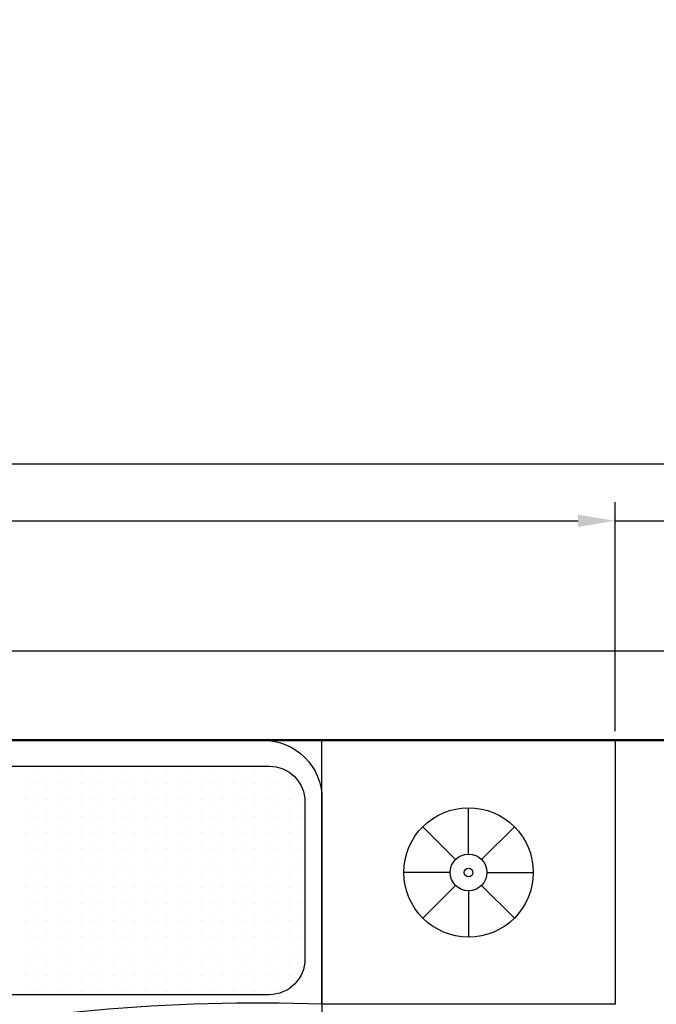
# Model space of a CAD drawing. Units: inches. Extents: x 3064 to 19385, y 846 to 15425.
# Tile 8 of 108: x 3469 to 3511, y 1373 to 1439. Entities that reach past the tile are written whole.
import ezdxf

# ---------------------------------------------------------------- set-up
doc = ezdxf.new("R2010")
doc.units = ezdxf.units.IN
for name, color, linetype, lineweight in [('A-ANNO-DIMS', 2, 'Continuous', 18), ('A-FLOR-FIXT', 9, 'Continuous', 18), ('A-WALL', 7, 'Continuous', 50), ('C-PROP', 6, 'Continuous', 25)]:
    doc.layers.add(name, color=color, linetype=linetype, lineweight=lineweight)
doc.layers.add('BLOCK', color=6, linetype='Continuous')
doc.styles.get("Standard").update_dxf_attribs({"font": 'arial.ttf'})
doc.dimstyles.new('ISO-25', dxfattribs={"dimtxt": 9, "dimasz": 2.5, "dimexe": 1.25, "dimexo": 0.625, "dimtad": 1, "dimdec": 1, "dimlunit": 3, "dimtxsty": 'Standard', "dimcen": 2.5, "dimadec": 0, "dimazin": 0, "dimtfac": 1, "dimtdec": 1, "dimtmove": 0, "dimatfit": 3, "dimfxl": 1, "dimarcsym": 0})

# ---------------------------------------------------------------- blocks, each defined once
blk = doc.blocks.new('*X7')
at = {"color": 0}
for p, q in [((275.4375, 457.03125), (275.4375, 457.03125)), ((275.625, 456.9375), (275.625, 456.9375)), ((275.8125, 457.03125), (275.8125, 457.03125)), ((276, 456.9375), (276, 456.9375)), ((276.1875, 457.03125), (276.1875, 457.03125)), ((276.375, 456.9375), (276.375, 456.9375)), ((276.5625, 457.03125), (276.5625, 457.03125)), ((276.75, 456.9375), (276.75, 456.9375)), ((276.9375, 457.03125), (276.9375, 457.03125)), ((277.125, 456.9375), (277.125, 456.9375)), ((277.3125, 457.03125), (277.3125, 457.03125)), ((277.5, 456.9375), (277.5, 456.9375)), ((277.6875, 457.03125), (277.6875, 457.03125)), ((277.875, 456.9375), (277.875, 456.9375)), ((278.0625, 457.03125), (278.0625, 457.03125)), ((278.25, 456.9375), (278.25, 456.9375)), ((278.4375, 457.03125), (278.4375, 457.03125)), ((278.625, 456.9375), (278.625, 456.9375)), ((278.8125, 457.03125), (278.8125, 457.03125)), ((279, 456.9375), (279, 456.9375)), ((279.1875, 457.03125), (279.1875, 457.03125)), ((279.375, 456.9375), (279.375, 456.9375)), ((279.5625, 457.03125), (279.5625, 457.03125)), ((279.75, 456.9375), (279.75, 456.9375)), ((275.4375, 456.84375), (275.4375, 456.84375)), ((275.625, 456.75), (275.625, 456.75)), ((275.8125, 456.84375), (275.8125, 456.84375)), ((276, 456.75), (276, 456.75)), ((276.1875, 456.84375), (276.1875, 456.84375)), ((276.375, 456.75), (276.375, 456.75)), ((276.5625, 456.84375), (276.5625, 456.84375)), ((276.75, 456.75), (276.75, 456.75)), ((276.9375, 456.84375), (276.9375, 456.84375)), ((277.125, 456.75), (277.125, 456.75)), ((277.3125, 456.84375), (277.3125, 456.84375)), ((277.5, 456.75), (277.5, 456.75)), ((277.6875, 456.84375), (277.6875, 456.84375)), ((277.875, 456.75), (277.875, 456.75)), ((278.0625, 456.84375), (278.0625, 456.84375)), ((278.25, 456.75), (278.25, 456.75)), ((278.4375, 456.84375), (278.4375, 456.84375)), ((278.625, 456.75), (278.625, 456.75)), ((278.8125, 456.84375), (278.8125, 456.84375)), ((279, 456.75), (279, 456.75)), ((279.1875, 456.84375), (279.1875, 456.84375)), ((279.375, 456.75), (279.375, 456.75)), ((279.5625, 456.84375), (279.5625, 456.84375)), ((279.75, 456.75), (279.75, 456.75)), ((279.9375, 456.84375), (279.9375, 456.84375)), ((280.125, 456.75), (280.125, 456.75)), ((275.4375, 456.65625), (275.4375, 456.65625)), ((275.625, 456.5625), (275.625, 456.5625)), ((275.8125, 456.65625), (275.8125, 456.65625)), ((276, 456.5625), (276, 456.5625)), ((276.1875, 456.65625), (276.1875, 456.65625)), ((276.375, 456.5625), (276.375, 456.5625)), ((276.5625, 456.65625), (276.5625, 456.65625)), ((276.75, 456.5625), (276.75, 456.5625)), ((276.9375, 456.65625), (276.9375, 456.65625)), ((277.125, 456.5625), (277.125, 456.5625)), ((277.3125, 456.65625), (277.3125, 456.65625)), ((277.5, 456.5625), (277.5, 456.5625)), ((277.6875, 456.65625), (277.6875, 456.65625)), ((277.875, 456.5625), (277.875, 456.5625)), ((278.0625, 456.65625), (278.0625, 456.65625)), ((278.25, 456.5625), (278.25, 456.5625)), ((278.4375, 456.65625), (278.4375, 456.65625)), ((278.625, 456.5625), (278.625, 456.5625)), ((278.8125, 456.65625), (278.8125, 456.65625)), ((279, 456.5625), (279, 456.5625)), ((279.1875, 456.65625), (279.1875, 456.65625)), ((279.375, 456.5625), (279.375, 456.5625)), ((279.5625, 456.65625), (279.5625, 456.65625)), ((279.75, 456.5625), (279.75, 456.5625)), ((279.9375, 456.65625), (279.9375, 456.65625)), ((280.125, 456.5625), (280.125, 456.5625)), ((275.4375, 456.46875), (275.4375, 456.46875)), ((275.625, 456.375), (275.625, 456.375)), ((275.8125, 456.46875), (275.8125, 456.46875)), ((276, 456.375), (276, 456.375)), ((276.1875, 456.46875), (276.1875, 456.46875)), ((276.375, 456.375), (276.375, 456.375)), ((276.5625, 456.46875), (276.5625, 456.46875)), ((276.75, 456.375), (276.75, 456.375)), ((276.9375, 456.46875), (276.9375, 456.46875)), ((277.125, 456.375), (277.125, 456.375)), ((277.3125, 456.46875), (277.3125, 456.46875)), ((277.5, 456.375), (277.5, 456.375)), ((277.6875, 456.46875), (277.6875, 456.46875)), ((277.875, 456.375), (277.875, 456.375)), ((278.0625, 456.46875), (278.0625, 456.46875)), ((278.25, 456.375), (278.25, 456.375)), ((278.4375, 456.46875), (278.4375, 456.46875)), ((278.625, 456.375), (278.625, 456.375)), ((278.8125, 456.46875), (278.8125, 456.46875)), ((279, 456.375), (279, 456.375)), ((279.1875, 456.46875), (279.1875, 456.46875)), ((279.375, 456.375), (279.375, 456.375)), ((279.5625, 456.46875), (279.5625, 456.46875)), ((279.75, 456.375), (279.75, 456.375)), ((279.9375, 456.46875), (279.9375, 456.46875)), ((280.125, 456.375), (280.125, 456.375)), ((275.4375, 456.28125), (275.4375, 456.28125)), ((275.8125, 456.28125), (275.8125, 456.28125)), ((276.1875, 456.28125), (276.1875, 456.28125)), ((276.5625, 456.28125), (276.5625, 456.28125)), ((276.9375, 456.28125), (276.9375, 456.28125)), ((277.3125, 456.28125), (277.3125, 456.28125)), ((277.6875, 456.28125), (277.6875, 456.28125)), ((278.0625, 456.28125), (278.0625, 456.28125)), ((278.4375, 456.28125), (278.4375, 456.28125)), ((278.8125, 456.28125), (278.8125, 456.28125)), ((279.1875, 456.28125), (279.1875, 456.28125)), ((279.5625, 456.28125), (279.5625, 456.28125)), ((279.9375, 456.28125), (279.9375, 456.28125)), ((275.4375, 456.09375), (275.4375, 456.09375)), ((275.625, 456.1875), (275.625, 456.1875)), ((275.8125, 456.09375), (275.8125, 456.09375)), ((276, 456.1875), (276, 456.1875)), ((276.1875, 456.09375), (276.1875, 456.09375)), ((276.375, 456.1875), (276.375, 456.1875)), ((276.5625, 456.09375), (276.5625, 456.09375)), ((276.75, 456.1875), (276.75, 456.1875)), ((276.9375, 456.09375), (276.9375, 456.09375)), ((277.125, 456.1875), (277.125, 456.1875)), ((277.3125, 456.09375), (277.3125, 456.09375)), ((277.5, 456.1875), (277.5, 456.1875)), ((277.6875, 456.09375), (277.6875, 456.09375)), ((277.875, 456.1875), (277.875, 456.1875)), ((278.0625, 456.09375), (278.0625, 456.09375)), ((278.25, 456.1875), (278.25, 456.1875)), ((278.4375, 456.09375), (278.4375, 456.09375)), ((278.625, 456.1875), (278.625, 456.1875)), ((278.8125, 456.09375), (278.8125, 456.09375)), ((279, 456.1875), (279, 456.1875)), ((279.1875, 456.09375), (279.1875, 456.09375)), ((279.375, 456.1875), (279.375, 456.1875)), ((279.5625, 456.09375), (279.5625, 456.09375)), ((279.75, 456.1875), (279.75, 456.1875)), ((279.9375, 456.09375), (279.9375, 456.09375)), ((280.125, 456.1875), (280.125, 456.1875)), ((275.4375, 455.90625), (275.4375, 455.90625)), ((275.625, 456), (275.625, 456)), ((275.8125, 455.90625), (275.8125, 455.90625)), ((276, 456), (276, 456)), ((276.1875, 455.90625), (276.1875, 455.90625)), ((276.375, 456), (276.375, 456)), ((276.5625, 455.90625), (276.5625, 455.90625)), ((276.75, 456), (276.75, 456)), ((276.9375, 455.90625), (276.9375, 455.90625)), ((277.125, 456), (277.125, 456)), ((277.3125, 455.90625), (277.3125, 455.90625)), ((277.5, 456), (277.5, 456)), ((277.6875, 455.90625), (277.6875, 455.90625)), ((277.875, 456), (277.875, 456)), ((278.0625, 455.90625), (278.0625, 455.90625)), ((278.25, 456), (278.25, 456)), ((278.4375, 455.90625), (278.4375, 455.90625)), ((278.625, 456), (278.625, 456)), ((278.8125, 455.90625), (278.8125, 455.90625)), ((279, 456), (279, 456)), ((279.1875, 455.90625), (279.1875, 455.90625)), ((279.375, 456), (279.375, 456)), ((279.5625, 455.90625), (279.5625, 455.90625)), ((279.75, 456), (279.75, 456)), ((279.9375, 455.90625), (279.9375, 455.90625)), ((280.125, 456), (280.125, 456)), ((275.4375, 455.71875), (275.4375, 455.71875)), ((275.625, 455.8125), (275.625, 455.8125)), ((275.8125, 455.71875), (275.8125, 455.71875)), ((276, 455.8125), (276, 455.8125)), ((276.1875, 455.71875), (276.1875, 455.71875)), ((276.375, 455.8125), (276.375, 455.8125)), ((276.5625, 455.71875), (276.5625, 455.71875)), ((276.75, 455.8125), (276.75, 455.8125)), ((276.9375, 455.71875), (276.9375, 455.71875)), ((277.125, 455.8125), (277.125, 455.8125)), ((277.3125, 455.71875), (277.3125, 455.71875)), ((277.5, 455.8125), (277.5, 455.8125)), ((277.6875, 455.71875), (277.6875, 455.71875)), ((277.875, 455.8125), (277.875, 455.8125)), ((278.0625, 455.71875), (278.0625, 455.71875)), ((278.25, 455.8125), (278.25, 455.8125)), ((278.4375, 455.71875), (278.4375, 455.71875)), ((278.625, 455.8125), (278.625, 455.8125)), ((278.8125, 455.71875), (278.8125, 455.71875)), ((279, 455.8125), (279, 455.8125)), ((279.1875, 455.71875), (279.1875, 455.71875)), ((279.375, 455.8125), (279.375, 455.8125)), ((279.5625, 455.71875), (279.5625, 455.71875)), ((279.75, 455.8125), (279.75, 455.8125)), ((279.9375, 455.71875), (279.9375, 455.71875)), ((280.125, 455.8125), (280.125, 455.8125)), ((275.4375, 455.53125), (275.4375, 455.53125)), ((275.625, 455.625), (275.625, 455.625)), ((275.8125, 455.53125), (275.8125, 455.53125)), ((276, 455.625), (276, 455.625)), ((276.1875, 455.53125), (276.1875, 455.53125)), ((276.375, 455.625), (276.375, 455.625)), ((276.5625, 455.53125), (276.5625, 455.53125)), ((276.75, 455.625), (276.75, 455.625)), ((276.9375, 455.53125), (276.9375, 455.53125)), ((277.125, 455.625), (277.125, 455.625)), ((277.3125, 455.53125), (277.3125, 455.53125)), ((277.5, 455.625), (277.5, 455.625)), ((277.6875, 455.53125), (277.6875, 455.53125)), ((277.875, 455.625), (277.875, 455.625)), ((278.0625, 455.53125), (278.0625, 455.53125)), ((278.25, 455.625), (278.25, 455.625)), ((278.4375, 455.53125), (278.4375, 455.53125)), ((278.625, 455.625), (278.625, 455.625)), ((278.8125, 455.53125), (278.8125, 455.53125)), ((279, 455.625), (279, 455.625)), ((279.1875, 455.53125), (279.1875, 455.53125)), ((279.375, 455.625), (279.375, 455.625)), ((279.5625, 455.53125), (279.5625, 455.53125)), ((279.75, 455.625), (279.75, 455.625)), ((279.9375, 455.53125), (279.9375, 455.53125)), ((280.125, 455.625), (280.125, 455.625)), ((275.625, 455.4375), (275.625, 455.4375)), ((276, 455.4375), (276, 455.4375)), ((276.375, 455.4375), (276.375, 455.4375)), ((276.75, 455.4375), (276.75, 455.4375)), ((277.125, 455.4375), (277.125, 455.4375)), ((277.5, 455.4375), (277.5, 455.4375)), ((277.875, 455.4375), (277.875, 455.4375)), ((278.25, 455.4375), (278.25, 455.4375)), ((278.625, 455.4375), (278.625, 455.4375)), ((279, 455.4375), (279, 455.4375)), ((279.375, 455.4375), (279.375, 455.4375)), ((279.75, 455.4375), (279.75, 455.4375)), ((280.125, 455.4375), (280.125, 455.4375)), ((275.4375, 455.34375), (275.4375, 455.34375)), ((275.625, 455.25), (275.625, 455.25)), ((275.8125, 455.34375), (275.8125, 455.34375)), ((276, 455.25), (276, 455.25)), ((276.1875, 455.34375), (276.1875, 455.34375)), ((276.375, 455.25), (276.375, 455.25)), ((276.5625, 455.34375), (276.5625, 455.34375)), ((276.75, 455.25), (276.75, 455.25)), ((276.9375, 455.34375), (276.9375, 455.34375)), ((277.125, 455.25), (277.125, 455.25)), ((277.3125, 455.34375), (277.3125, 455.34375)), ((277.5, 455.25), (277.5, 455.25)), ((277.6875, 455.34375), (277.6875, 455.34375)), ((277.875, 455.25), (277.875, 455.25)), ((278.0625, 455.34375), (278.0625, 455.34375)), ((278.25, 455.25), (278.25, 455.25)), ((278.4375, 455.34375), (278.4375, 455.34375)), ((278.625, 455.25), (278.625, 455.25)), ((278.8125, 455.34375), (278.8125, 455.34375)), ((279, 455.25), (279, 455.25)), ((279.1875, 455.34375), (279.1875, 455.34375)), ((279.375, 455.25), (279.375, 455.25)), ((279.5625, 455.34375), (279.5625, 455.34375)), ((279.75, 455.25), (279.75, 455.25)), ((279.9375, 455.34375), (279.9375, 455.34375)), ((280.125, 455.25), (280.125, 455.25)), ((275.4375, 455.15625), (275.4375, 455.15625)), ((275.625, 455.0625), (275.625, 455.0625)), ((275.8125, 455.15625), (275.8125, 455.15625)), ((276, 455.0625), (276, 455.0625)), ((276.1875, 455.15625), (276.1875, 455.15625)), ((276.375, 455.0625), (276.375, 455.0625)), ((276.5625, 455.15625), (276.5625, 455.15625)), ((276.75, 455.0625), (276.75, 455.0625)), ((276.9375, 455.15625), (276.9375, 455.15625)), ((277.125, 455.0625), (277.125, 455.0625)), ((277.3125, 455.15625), (277.3125, 455.15625)), ((277.5, 455.0625), (277.5, 455.0625)), ((277.6875, 455.15625), (277.6875, 455.15625)), ((277.875, 455.0625), (277.875, 455.0625)), ((278.0625, 455.15625), (278.0625, 455.15625)), ((278.25, 455.0625), (278.25, 455.0625)), ((278.4375, 455.15625), (278.4375, 455.15625)), ((278.625, 455.0625), (278.625, 455.0625)), ((278.8125, 455.15625), (278.8125, 455.15625)), ((279, 455.0625), (279, 455.0625)), ((279.1875, 455.15625), (279.1875, 455.15625)), ((279.375, 455.0625), (279.375, 455.0625)), ((279.5625, 455.15625), (279.5625, 455.15625)), ((279.75, 455.0625), (279.75, 455.0625)), ((279.9375, 455.15625), (279.9375, 455.15625)), ((280.125, 455.0625), (280.125, 455.0625)), ((275.4375, 454.96875), (275.4375, 454.96875)), ((275.625, 454.875), (275.625, 454.875)), ((275.8125, 454.96875), (275.8125, 454.96875)), ((276, 454.875), (276, 454.875)), ((276.1875, 454.96875), (276.1875, 454.96875)), ((276.375, 454.875), (276.375, 454.875)), ((276.5625, 454.96875), (276.5625, 454.96875)), ((276.75, 454.875), (276.75, 454.875)), ((276.9375, 454.96875), (276.9375, 454.96875)), ((277.125, 454.875), (277.125, 454.875)), ((277.3125, 454.96875), (277.3125, 454.96875)), ((277.5, 454.875), (277.5, 454.875)), ((277.6875, 454.96875), (277.6875, 454.96875)), ((277.875, 454.875), (277.875, 454.875)), ((278.0625, 454.96875), (278.0625, 454.96875)), ((278.25, 454.875), (278.25, 454.875)), ((278.4375, 454.96875), (278.4375, 454.96875)), ((278.625, 454.875), (278.625, 454.875)), ((278.8125, 454.96875), (278.8125, 454.96875)), ((279, 454.875), (279, 454.875)), ((279.1875, 454.96875), (279.1875, 454.96875)), ((279.375, 454.875), (279.375, 454.875)), ((279.5625, 454.96875), (279.5625, 454.96875)), ((279.75, 454.875), (279.75, 454.875)), ((279.9375, 454.96875), (279.9375, 454.96875)), ((280.125, 454.875), (280.125, 454.875)), ((275.4375, 454.78125), (275.4375, 454.78125)), ((275.625, 454.6875), (275.625, 454.6875)), ((275.8125, 454.78125), (275.8125, 454.78125)), ((276, 454.6875), (276, 454.6875)), ((276.1875, 454.78125), (276.1875, 454.78125)), ((276.375, 454.6875), (276.375, 454.6875)), ((276.5625, 454.78125), (276.5625, 454.78125)), ((276.75, 454.6875), (276.75, 454.6875)), ((276.9375, 454.78125), (276.9375, 454.78125)), ((277.125, 454.6875), (277.125, 454.6875)), ((277.3125, 454.78125), (277.3125, 454.78125)), ((277.5, 454.6875), (277.5, 454.6875)), ((277.6875, 454.78125), (277.6875, 454.78125)), ((277.875, 454.6875), (277.875, 454.6875)), ((278.0625, 454.78125), (278.0625, 454.78125)), ((278.25, 454.6875), (278.25, 454.6875)), ((278.4375, 454.78125), (278.4375, 454.78125)), ((278.625, 454.6875), (278.625, 454.6875)), ((278.8125, 454.78125), (278.8125, 454.78125)), ((279, 454.6875), (279, 454.6875)), ((279.1875, 454.78125), (279.1875, 454.78125)), ((279.375, 454.6875), (279.375, 454.6875)), ((279.5625, 454.78125), (279.5625, 454.78125)), ((279.75, 454.6875), (279.75, 454.6875)), ((279.9375, 454.78125), (279.9375, 454.78125)), ((280.125, 454.6875), (280.125, 454.6875)), ((275.4375, 454.59375), (275.4375, 454.59375)), ((275.8125, 454.59375), (275.8125, 454.59375)), ((276.1875, 454.59375), (276.1875, 454.59375)), ((276.5625, 454.59375), (276.5625, 454.59375)), ((276.9375, 454.59375), (276.9375, 454.59375)), ((277.3125, 454.59375), (277.3125, 454.59375)), ((277.6875, 454.59375), (277.6875, 454.59375)), ((278.0625, 454.59375), (278.0625, 454.59375)), ((278.4375, 454.59375), (278.4375, 454.59375)), ((278.8125, 454.59375), (278.8125, 454.59375)), ((279.1875, 454.59375), (279.1875, 454.59375)), ((279.5625, 454.59375), (279.5625, 454.59375)), ((279.9375, 454.59375), (279.9375, 454.59375)), ((275.4375, 454.40625), (275.4375, 454.40625)), ((275.625, 454.5), (275.625, 454.5)), ((275.8125, 454.40625), (275.8125, 454.40625)), ((276, 454.5), (276, 454.5)), ((276.1875, 454.40625), (276.1875, 454.40625)), ((276.375, 454.5), (276.375, 454.5)), ((276.5625, 454.40625), (276.5625, 454.40625)), ((276.75, 454.5), (276.75, 454.5)), ((276.9375, 454.40625), (276.9375, 454.40625)), ((277.125, 454.5), (277.125, 454.5)), ((277.3125, 454.40625), (277.3125, 454.40625)), ((277.5, 454.5), (277.5, 454.5)), ((277.6875, 454.40625), (277.6875, 454.40625)), ((277.875, 454.5), (277.875, 454.5)), ((278.0625, 454.40625), (278.0625, 454.40625)), ((278.25, 454.5), (278.25, 454.5)), ((278.4375, 454.40625), (278.4375, 454.40625)), ((278.625, 454.5), (278.625, 454.5)), ((278.8125, 454.40625), (278.8125, 454.40625)), ((279, 454.5), (279, 454.5)), ((279.1875, 454.40625), (279.1875, 454.40625)), ((279.375, 454.5), (279.375, 454.5)), ((279.5625, 454.40625), (279.5625, 454.40625)), ((279.75, 454.5), (279.75, 454.5)), ((279.9375, 454.40625), (279.9375, 454.40625)), ((280.125, 454.5), (280.125, 454.5)), ((275.4375, 454.21875), (275.4375, 454.21875)), ((275.625, 454.3125), (275.625, 454.3125)), ((275.8125, 454.21875), (275.8125, 454.21875)), ((276, 454.3125), (276, 454.3125)), ((276.1875, 454.21875), (276.1875, 454.21875)), ((276.375, 454.3125), (276.375, 454.3125)), ((276.5625, 454.21875), (276.5625, 454.21875)), ((276.75, 454.3125), (276.75, 454.3125)), ((276.9375, 454.21875), (276.9375, 454.21875)), ((277.125, 454.3125), (277.125, 454.3125)), ((277.3125, 454.21875), (277.3125, 454.21875)), ((277.5, 454.3125), (277.5, 454.3125)), ((277.6875, 454.21875), (277.6875, 454.21875)), ((277.875, 454.3125), (277.875, 454.3125)), ((278.0625, 454.21875), (278.0625, 454.21875)), ((278.25, 454.3125), (278.25, 454.3125)), ((278.4375, 454.21875), (278.4375, 454.21875)), ((278.625, 454.3125), (278.625, 454.3125)), ((278.8125, 454.21875), (278.8125, 454.21875)), ((279, 454.3125), (279, 454.3125)), ((279.1875, 454.21875), (279.1875, 454.21875)), ((279.375, 454.3125), (279.375, 454.3125)), ((279.5625, 454.21875), (279.5625, 454.21875)), ((279.75, 454.3125), (279.75, 454.3125)), ((279.9375, 454.21875), (279.9375, 454.21875)), ((280.125, 454.3125), (280.125, 454.3125)), ((275.4375, 454.03125), (275.4375, 454.03125)), ((275.625, 454.125), (275.625, 454.125)), ((275.8125, 454.03125), (275.8125, 454.03125)), ((276, 454.125), (276, 454.125)), ((276.1875, 454.03125), (276.1875, 454.03125)), ((276.375, 454.125), (276.375, 454.125)), ((276.5625, 454.03125), (276.5625, 454.03125)), ((276.75, 454.125), (276.75, 454.125)), ((276.9375, 454.03125), (276.9375, 454.03125)), ((277.125, 454.125), (277.125, 454.125)), ((277.3125, 454.03125), (277.3125, 454.03125)), ((277.5, 454.125), (277.5, 454.125)), ((277.6875, 454.03125), (277.6875, 454.03125)), ((277.875, 454.125), (277.875, 454.125)), ((278.0625, 454.03125), (278.0625, 454.03125)), ((278.25, 454.125), (278.25, 454.125)), ((278.4375, 454.03125), (278.4375, 454.03125)), ((278.625, 454.125), (278.625, 454.125)), ((278.8125, 454.03125), (278.8125, 454.03125)), ((279, 454.125), (279, 454.125)), ((279.1875, 454.03125), (279.1875, 454.03125)), ((279.375, 454.125), (279.375, 454.125)), ((279.5625, 454.03125), (279.5625, 454.03125)), ((279.75, 454.125), (279.75, 454.125)), ((279.9375, 454.03125), (279.9375, 454.03125)), ((280.125, 454.125), (280.125, 454.125)), ((275.625, 453.9375), (275.625, 453.9375)), ((276, 453.9375), (276, 453.9375)), ((276.375, 453.9375), (276.375, 453.9375)), ((276.75, 453.9375), (276.75, 453.9375)), ((277.125, 453.9375), (277.125, 453.9375)), ((277.5, 453.9375), (277.5, 453.9375)), ((277.875, 453.9375), (277.875, 453.9375)), ((278.25, 453.9375), (278.25, 453.9375)), ((278.625, 453.9375), (278.625, 453.9375)), ((279, 453.9375), (279, 453.9375)), ((279.375, 453.9375), (279.375, 453.9375)), ((279.75, 453.9375), (279.75, 453.9375)), ((280.125, 453.9375), (280.125, 453.9375)), ((275.4375, 453.84375), (275.4375, 453.84375)), ((275.625, 453.75), (275.625, 453.75)), ((275.8125, 453.84375), (275.8125, 453.84375)), ((276, 453.75), (276, 453.75)), ((276.1875, 453.84375), (276.1875, 453.84375)), ((276.375, 453.75), (276.375, 453.75)), ((276.5625, 453.84375), (276.5625, 453.84375)), ((276.75, 453.75), (276.75, 453.75)), ((276.9375, 453.84375), (276.9375, 453.84375)), ((277.125, 453.75), (277.125, 453.75)), ((277.3125, 453.84375), (277.3125, 453.84375)), ((277.5, 453.75), (277.5, 453.75)), ((277.6875, 453.84375), (277.6875, 453.84375)), ((277.875, 453.75), (277.875, 453.75)), ((278.0625, 453.84375), (278.0625, 453.84375)), ((278.25, 453.75), (278.25, 453.75)), ((278.4375, 453.84375), (278.4375, 453.84375)), ((278.625, 453.75), (278.625, 453.75)), ((278.8125, 453.84375), (278.8125, 453.84375)), ((279, 453.75), (279, 453.75)), ((279.1875, 453.84375), (279.1875, 453.84375)), ((279.375, 453.75), (279.375, 453.75)), ((279.5625, 453.84375), (279.5625, 453.84375)), ((279.75, 453.75), (279.75, 453.75)), ((279.9375, 453.84375), (279.9375, 453.84375)), ((280.125, 453.75), (280.125, 453.75)), ((275.4375, 453.65625), (275.4375, 453.65625)), ((275.625, 453.5625), (275.625, 453.5625)), ((275.8125, 453.65625), (275.8125, 453.65625)), ((276, 453.5625), (276, 453.5625)), ((276.1875, 453.65625), (276.1875, 453.65625)), ((276.375, 453.5625), (276.375, 453.5625)), ((276.5625, 453.65625), (276.5625, 453.65625)), ((276.75, 453.5625), (276.75, 453.5625)), ((276.9375, 453.65625), (276.9375, 453.65625)), ((277.125, 453.5625), (277.125, 453.5625)), ((277.3125, 453.65625), (277.3125, 453.65625)), ((277.5, 453.5625), (277.5, 453.5625)), ((277.6875, 453.65625), (277.6875, 453.65625)), ((277.875, 453.5625), (277.875, 453.5625)), ((278.0625, 453.65625), (278.0625, 453.65625)), ((278.25, 453.5625), (278.25, 453.5625)), ((278.4375, 453.65625), (278.4375, 453.65625)), ((278.625, 453.5625), (278.625, 453.5625)), ((278.8125, 453.65625), (278.8125, 453.65625)), ((279, 453.5625), (279, 453.5625)), ((279.1875, 453.65625), (279.1875, 453.65625)), ((279.375, 453.5625), (279.375, 453.5625)), ((279.5625, 453.65625), (279.5625, 453.65625)), ((279.75, 453.5625), (279.75, 453.5625)), ((279.9375, 453.65625), (279.9375, 453.65625)), ((280.125, 453.5625), (280.125, 453.5625)), ((275.4375, 453.46875), (275.4375, 453.46875)), ((275.625, 453.375), (275.625, 453.375)), ((275.8125, 453.46875), (275.8125, 453.46875)), ((276, 453.375), (276, 453.375)), ((276.1875, 453.46875), (276.1875, 453.46875)), ((276.375, 453.375), (276.375, 453.375)), ((276.5625, 453.46875), (276.5625, 453.46875)), ((276.75, 453.375), (276.75, 453.375)), ((276.9375, 453.46875), (276.9375, 453.46875)), ((277.125, 453.375), (277.125, 453.375)), ((277.3125, 453.46875), (277.3125, 453.46875)), ((277.5, 453.375), (277.5, 453.375)), ((277.6875, 453.46875), (277.6875, 453.46875)), ((277.875, 453.375), (277.875, 453.375)), ((278.0625, 453.46875), (278.0625, 453.46875)), ((278.25, 453.375), (278.25, 453.375)), ((278.4375, 453.46875), (278.4375, 453.46875)), ((278.625, 453.375), (278.625, 453.375)), ((278.8125, 453.46875), (278.8125, 453.46875)), ((279, 453.375), (279, 453.375)), ((279.1875, 453.46875), (279.1875, 453.46875)), ((279.375, 453.375), (279.375, 453.375)), ((279.5625, 453.46875), (279.5625, 453.46875)), ((279.75, 453.375), (279.75, 453.375)), ((279.9375, 453.46875), (279.9375, 453.46875)), ((275.4375, 453.28125), (275.4375, 453.28125)), ((275.625, 453.1875), (275.625, 453.1875)), ((275.8125, 453.28125), (275.8125, 453.28125)), ((276, 453.1875), (276, 453.1875)), ((276.1875, 453.28125), (276.1875, 453.28125)), ((276.375, 453.1875), (276.375, 453.1875)), ((276.5625, 453.28125), (276.5625, 453.28125)), ((276.75, 453.1875), (276.75, 453.1875)), ((276.9375, 453.28125), (276.9375, 453.28125)), ((277.125, 453.1875), (277.125, 453.1875)), ((277.3125, 453.28125), (277.3125, 453.28125)), ((277.5, 453.1875), (277.5, 453.1875)), ((277.6875, 453.28125), (277.6875, 453.28125)), ((277.875, 453.1875), (277.875, 453.1875)), ((278.0625, 453.28125), (278.0625, 453.28125)), ((278.25, 453.1875), (278.25, 453.1875)), ((278.4375, 453.28125), (278.4375, 453.28125)), ((278.625, 453.1875), (278.625, 453.1875)), ((278.8125, 453.28125), (278.8125, 453.28125)), ((279, 453.1875), (279, 453.1875)), ((279.1875, 453.28125), (279.1875, 453.28125)), ((279.375, 453.1875), (279.375, 453.1875)), ((279.5625, 453.28125), (279.5625, 453.28125)), ((279.75, 453.1875), (279.75, 453.1875)), ((279.9375, 453.28125), (279.9375, 453.28125))]:
    blk.add_line(p, q, dxfattribs=at)
blk = doc.blocks.new('A$C52E67D0D')
at = {"layer": 'BLOCK'}
for p, q in [((2251.5, 1605.5), (2251.5, 1684.7)), ((2229.3, 1596.3), (2173.3, 1652.3)), ((2273.7, 1596.3), (2329.7, 1652.3)), ((2220.1, 1574.1), (2140.9, 1574.1)), ((2282.9, 1574.1), (2362.1, 1574.1)), ((2229.3, 1551.9), (2173.3, 1495.9)), ((2273.7, 1551.9), (2329.7, 1495.9)), ((2251.5, 1542.8), (2251.5, 1463.5))]:
    blk.add_line(p, q, dxfattribs=at)
for points in [[(1901, 0), (601, 0, -0.414214), (501, 100), (501, 1700, -0.414214), (601, 1800), (1901, 1800, -0.414214), (2001, 1700), (2001, 100, -0.414214)], [(1911, 1365.1), (1335, 1365.1, -0.414214), (1274.2, 1425.9), (1274.2, 1694.8, -0.414214), (1335, 1755.7), (1911, 1755.7, -0.414214), (1971.8, 1694.8), (1971.8, 1425.9, -0.414214)]]:
    blk.add_lwpolyline(points, format="xyb", close=True, dxfattribs=at)
blk.add_lwpolyline([(2001, 1348.6), (2001, 1799.6), (2502, 1799.6), (2502, 1348.6)], close=True, dxfattribs=at)
for radius in [110.6, 31.4, 7.46]:
    blk.add_circle((2251.5, 1574.1), radius, dxfattribs=at)
blk.add_arc((1888.6, -1664.5), 3015.3, 87.8642, 117.4001, dxfattribs=at)
at = {"layer": 'BLOCK', "xscale": 100, "yscale": 100, "zscale": 100}
blk.add_blockref('*X7', (-26050, -43948.2), dxfattribs=at)
blk = doc.blocks.new('*D38')
at = {"layer": 'A-ANNO-DIMS', "color": 0, "lineweight": -2, "transparency": 16777216}
for p, q in [((3220.848, 1396.965), (3220.848, 1410.198)), ((3562.848, 1396.965), (3562.848, 1410.198)), ((3223.348, 1408.948), (3560.348, 1408.948))]:
    blk.add_line(p, q, dxfattribs=at)
at = {"layer": 'A-ANNO-DIMS', "color": 0, "transparency": 16777216}
for points in [[(3223.348, 1409.365), (3223.348, 1408.531), (3220.848, 1408.948)], [(3560.348, 1409.365), (3560.348, 1408.531), (3562.848, 1408.948)]]:
    blk.add_solid(points, dxfattribs=at)
at = {"layer": 'Defpoints', "color": 0, "transparency": 16777216}
for p in [(3562.848, 1408.948), (3220.848, 1396.34), (3562.848, 1396.34)]:
    blk.add_point(p, dxfattribs=at)
at = {"layer": 'A-ANNO-DIMS', "color": 0, "transparency": 16777216, "insert": (3391.848, 1414.168), "char_height": 9, "attachment_point": 5}
blk.add_mtext('28\'-6"', dxfattribs=at)
blk = doc.blocks.new('*D401')
at = {"layer": 'A-ANNO-DIMS', "color": 0, "lineweight": -2, "transparency": 16777216}
for p, q in [((3410.096, 1390.965), (3410.096, 1406.366)), ((3508.6, 1390.965), (3508.6, 1406.366)), ((3412.596, 1405.116), (3506.1, 1405.116)), ((3508.6, 1405.116), (3617.127, 1405.116))]:
    blk.add_line(p, q, dxfattribs=at)
at = {"layer": 'A-ANNO-DIMS', "color": 0, "transparency": 16777216}
for points in [[(3412.596, 1405.532), (3412.596, 1404.699), (3410.096, 1405.116)], [(3506.1, 1405.532), (3506.1, 1404.699), (3508.6, 1405.116)]]:
    blk.add_solid(points, dxfattribs=at)
at = {"layer": 'Defpoints', "color": 0, "transparency": 16777216}
for p in [(3508.6, 1405.116), (3410.096, 1390.34), (3508.6, 1390.34)]:
    blk.add_point(p, dxfattribs=at)
at = {"layer": 'A-ANNO-DIMS', "color": 0, "transparency": 16777216, "insert": (3564.114, 1410.394), "char_height": 9, "attachment_point": 5}
blk.add_mtext('BED 8\'-2 1/2" TYP.', dxfattribs=at)

msp = doc.modelspace()

# ---------------------------------------------------------------- linework, layer by layer
at = {"layer": 'A-WALL'}
msp.add_line((3556.848, 1390.34), (3361.848, 1390.34), dxfattribs=at)
at = {"layer": 'C-PROP'}
msp.add_line((3562.848, 1396.34), (3220.848, 1396.34), dxfattribs=at)

# ---------------------------------------------------------------- block references
at = {"layer": 'A-FLOR-FIXT', "xscale": 0.039370099999992, "yscale": 0.039370099999992, "zscale": 0.039370099999992}
msp.add_blockref('A$C52E67D0D', (3410.096, 1319.474), dxfattribs=at)

# ---------------------------------------------------------------- dimensions: what is measured, and where the dimension line sits
at = {"layer": 'A-ANNO-DIMS'}
dim = msp.add_linear_dim(base=(3508.6, 1405.116), p1=(3410.096, 1390.34), p2=(3508.6, 1390.34), text='BED <> TYP.', dimstyle='ISO-25', override={"dimdec": 1, "dimrnd": 0, "dimzin": 1, "dimlunit": 4, "dimfrac": 2}, dxfattribs=at)
dim.commit()
dim.dimension.update_dxf_attribs({"geometry": '*D401', "text_midpoint": (3564.114, 1410.394)})
dim = msp.add_linear_dim(base=(3562.848, 1408.948), p1=(3220.848, 1396.34), p2=(3562.848, 1396.34), dimstyle='ISO-25', override={"dimclrd": 0, "dimclre": 0, "dimclrt": 0}, dxfattribs=at)
dim.commit()
dim.dimension.update_dxf_attribs({"geometry": '*D38', "text_midpoint": (3391.848, 1414.168)})

doc.saveas('drawing.dxf')
